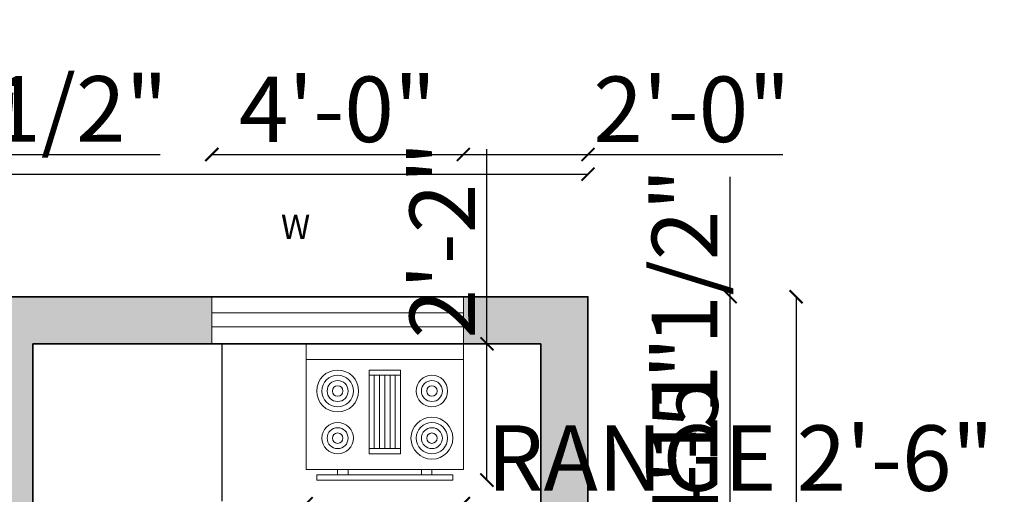
# Model space of a CAD drawing. Units: inches. Extents: x 1750 to 7466, y 1409 to 2004.
# Tile 5 of 5: x 1986 to 2174, y 1890 to 1981. Entities that reach past the tile are written whole.
import ezdxf

# ---------------------------------------------------------------- set-up
doc = ezdxf.new("R2010")
doc.units = ezdxf.units.IN
for name, color, linetype, lineweight in [('A-ANNO-DIMS', 2, 'Continuous', 18), ('A-ANNO-TEXT', 7, 'Continuous', 18), ('A-EQPM', 9, 'Continuous', 18), ('A-FLOR-CASE', 8, 'Continuous', 25), ('A-WALL', 7, 'Continuous', 35), ('WINDOW', 4, 'Continuous', 18)]:
    doc.layers.add(name, color=color, linetype=linetype, lineweight=lineweight)
doc.layers.add('A-WALL-PATT', color=18, linetype='Continuous', lineweight=13, true_color=0x000000)
doc.styles.get("Standard").update_dxf_attribs({"font": 'arial.ttf'})
doc.dimstyles.new('ISO-25', dxfattribs={"dimtxt": 12.5, "dimasz": 2.5, "dimexe": 1.25, "dimexo": 0.625, "dimtad": 1, "dimdec": 0, "dimlunit": 4, "dimtxsty": 'Standard', "dimblk": 'ARCHTICK', "dimcen": 2.5, "dimse1": 1, "dimse2": 1, "dimclrd": 2, "dimadec": 0, "dimazin": 0, "dimtfac": 1, "dimtdec": 0, "dimtmove": 0, "dimatfit": 3, "dimfxl": 1, "dimarcsym": 0})

# ---------------------------------------------------------------- blocks, each defined once
blk = doc.blocks.new('Range-Oven - 30 in top')
for p, q in [((0, -3), (30, -3)), ((12, -6), (18, -6)), ((13, -20), (13, -6)), ((14, -6), (14, -20)), ((15, -20), (15, -6)), ((16, -6), (16, -20)), ((17, -20), (17, -6)), ((18, -20), (12, -20)), ((6, -24), (6, -25)), ((8, -25), (8, -24)), ((22, -25), (22, -24)), ((24, -24), (24, -25))]:
    blk.add_line(p, q)
for points in [[(0, -24), (0, 0), (30, 0), (30, -24)], [(12, -21), (12, -5), (18, -5), (18, -21)], [(2, -26), (2, -25), (28, -25), (28, -26)]]:
    blk.add_lwpolyline(points, close=True)
for centre, radius in [((6, -9), 4), ((6, -9), 3), ((6, -9), 2), ((24, -9), 3), ((24, -9), 2), ((6, -9), 1), ((24, -9), 1), ((6, -18), 3), ((24, -18), 4), ((24, -18), 3), ((6, -18), 2), ((24, -18), 2), ((6, -18), 1), ((24, -18), 1)]:
    blk.add_circle(centre, radius)
blk = doc.blocks.new('_ArchTick')
at = {"color": 0, "linetype": 'ByBlock', "const_width": 0.15}
blk.add_lwpolyline([(-0.5, -0.5), (0.5, 0.5)], dxfattribs=at)
blk = doc.blocks.new('*D13')
at = {"layer": 'A-ANNO-DIMS', "color": 0, "lineweight": -2, "transparency": 16777216}
blk.add_line((1854.13, 1951.57), (2094.13, 1951.57), dxfattribs=at)
at = {"layer": 'Defpoints', "color": 0, "transparency": 16777216}
for p in [(2094.13, 1951.57), (1854.13, 1928.17), (2094.13, 1928.17)]:
    blk.add_point(p, dxfattribs=at)
at = {"layer": 'A-ANNO-DIMS', "color": 0, "lineweight": -2, "transparency": 16777216, "xscale": 2.5, "yscale": 2.5, "zscale": 2.5, "rotation": 180}
blk.add_blockref('_ArchTick', (1854.13, 1951.57), dxfattribs=at)
at = {"layer": 'A-ANNO-DIMS', "color": 0, "lineweight": -2, "transparency": 16777216, "xscale": 2.5, "yscale": 2.5, "zscale": 2.5}
blk.add_blockref('_ArchTick', (2094.13, 1951.57), dxfattribs=at)
at = {"layer": 'A-ANNO-DIMS', "color": 0, "transparency": 16777216, "insert": (1974.13, 1958.58), "char_height": 12.5, "attachment_point": 5}
blk.add_mtext("20'", dxfattribs=at)
blk = doc.blocks.new('*D14')
at = {"layer": 'A-ANNO-DIMS', "color": 0, "lineweight": -2, "transparency": 16777216}
blk.add_line((2133.87, 1928.17), (2133.87, 1448.17), dxfattribs=at)
at = {"layer": 'Defpoints', "color": 0, "transparency": 16777216}
for p in [(2094.13, 1928.17), (2094.13, 1448.17), (2133.87, 1448.17)]:
    blk.add_point(p, dxfattribs=at)
at = {"layer": 'A-ANNO-DIMS', "color": 0, "lineweight": -2, "transparency": 16777216, "xscale": 2.5, "yscale": 2.5, "zscale": 2.5}
for p, rotation in [((2133.87, 1928.17), 90), ((2133.87, 1448.17), 270)]:
    blk.add_blockref('_ArchTick', p, dxfattribs=dict(at, rotation=rotation))
at = {"layer": 'A-ANNO-DIMS', "color": 0, "transparency": 16777216, "insert": (2126.86, 1688.17), "char_height": 12.5, "attachment_point": 5, "rotation": 90}
blk.add_mtext("40'", dxfattribs=at)
blk = doc.blocks.new('*D19')
at = {"layer": 'A-ANNO-DIMS', "color": 2, "lineweight": -2, "transparency": 16777216}
for p, q in [((2040.34, 1888.67), (2070.34, 1888.67)), ((2070.34, 1888.67), (2173.62, 1888.67))]:
    blk.add_line(p, q, dxfattribs=at)
at = {"layer": 'Defpoints', "color": 0, "transparency": 16777216}
for p in [(2040.34, 1893.17), (2070.34, 1893.17), (2070.34, 1888.67)]:
    blk.add_point(p, dxfattribs=at)
at = {"layer": 'A-ANNO-DIMS', "color": 2, "lineweight": -2, "transparency": 16777216, "xscale": 2.5, "yscale": 2.5, "zscale": 2.5, "rotation": 180}
blk.add_blockref('_ArchTick', (2040.34, 1888.67), dxfattribs=at)
at = {"layer": 'A-ANNO-DIMS', "color": 2, "lineweight": -2, "transparency": 16777216, "xscale": 2.5, "yscale": 2.5, "zscale": 2.5}
blk.add_blockref('_ArchTick', (2070.34, 1888.67), dxfattribs=at)
at = {"layer": 'A-ANNO-DIMS', "color": 0, "transparency": 16777216, "insert": (2123.23, 1895.75), "char_height": 12.5, "attachment_point": 5}
blk.add_mtext('RANGE 2\'-6"', dxfattribs=at)
blk = doc.blocks.new('*D20')
at = {"layer": 'A-ANNO-DIMS', "color": 2, "lineweight": -2, "transparency": 16777216}
for p, q in [((2074.84, 1919.17), (2074.84, 1956.36)), ((2074.84, 1893.17), (2074.84, 1919.17))]:
    blk.add_line(p, q, dxfattribs=at)
at = {"layer": 'Defpoints', "color": 0, "transparency": 16777216}
for p in [(2070.34, 1919.17), (2074.84, 1919.17), (2070.34, 1893.17)]:
    blk.add_point(p, dxfattribs=at)
at = {"layer": 'A-ANNO-DIMS', "color": 2, "lineweight": -2, "transparency": 16777216, "xscale": 2.5, "yscale": 2.5, "zscale": 2.5}
for p, rotation in [((2074.84, 1919.17), 90), ((2074.84, 1893.17), 270)]:
    blk.add_blockref('_ArchTick', p, dxfattribs=dict(at, rotation=rotation))
at = {"layer": 'A-ANNO-DIMS', "color": 0, "transparency": 16777216, "insert": (2067.94, 1939.01), "char_height": 12.5, "attachment_point": 5, "rotation": 90}
blk.add_mtext('2\'-2"', dxfattribs=at)
blk = doc.blocks.new('*D39')
at = {"layer": 'A-ANNO-DIMS', "color": 2, "lineweight": -2, "transparency": 16777216}
for p, q in [((1775.98, 1919.17), (1775.98, 1889.13)), ((1775.98, 1889.13), (1775.98, 1851.94))]:
    blk.add_line(p, q, dxfattribs=at)
at = {"layer": 'Defpoints', "color": 0, "transparency": 16777216}
for p in [(2024.28, 1919.17), (1775.98, 1889.13), (2024.28, 1889.13)]:
    blk.add_point(p, dxfattribs=at)
at = {"layer": 'A-ANNO-DIMS', "color": 2, "lineweight": -2, "transparency": 16777216, "xscale": 2.5, "yscale": 2.5, "zscale": 2.5}
for p, rotation in [((1775.98, 1919.17), 90), ((1775.98, 1889.13), 270)]:
    blk.add_blockref('_ArchTick', p, dxfattribs=dict(at, rotation=rotation))
at = {"layer": 'A-ANNO-DIMS', "color": 0, "transparency": 16777216, "insert": (1768.98, 1869.28), "char_height": 12.5, "attachment_point": 5, "rotation": 90}
blk.add_mtext('2\'-6"', dxfattribs=at)
blk = doc.blocks.new('*D42')
at = {"layer": 'A-ANNO-DIMS', "color": 2, "lineweight": -2, "transparency": 16777216}
blk.add_line((2022.32, 1955.32), (2070.34, 1955.32), dxfattribs=at)
at = {"layer": 'Defpoints', "color": 0, "transparency": 16777216}
for p in [(2070.34, 1955.32), (2022.32, 1928.17), (2070.34, 1928.17)]:
    blk.add_point(p, dxfattribs=at)
at = {"layer": 'A-ANNO-DIMS', "color": 2, "lineweight": -2, "transparency": 16777216, "xscale": 2.5, "yscale": 2.5, "zscale": 2.5, "rotation": 180}
blk.add_blockref('_ArchTick', (2022.32, 1955.32), dxfattribs=at)
at = {"layer": 'A-ANNO-DIMS', "color": 2, "lineweight": -2, "transparency": 16777216, "xscale": 2.5, "yscale": 2.5, "zscale": 2.5}
blk.add_blockref('_ArchTick', (2070.34, 1955.32), dxfattribs=at)
at = {"layer": 'A-ANNO-DIMS', "color": 0, "transparency": 16777216, "insert": (2046.33, 1962.32), "char_height": 12.5, "attachment_point": 5}
blk.add_mtext('4\'-0"', dxfattribs=at)
blk = doc.blocks.new('*D43')
at = {"layer": 'A-ANNO-DIMS', "color": 2, "lineweight": -2, "transparency": 16777216}
for p, q in [((2070.34, 1955.32), (2094.13, 1955.32)), ((2094.13, 1955.32), (2131.32, 1955.32))]:
    blk.add_line(p, q, dxfattribs=at)
at = {"layer": 'Defpoints', "color": 0, "transparency": 16777216}
for p in [(2094.13, 1955.32), (2070.34, 1928.17), (2094.13, 1928.17)]:
    blk.add_point(p, dxfattribs=at)
at = {"layer": 'A-ANNO-DIMS', "color": 2, "lineweight": -2, "transparency": 16777216, "xscale": 2.5, "yscale": 2.5, "zscale": 2.5, "rotation": 180}
blk.add_blockref('_ArchTick', (2070.34, 1955.32), dxfattribs=at)
at = {"layer": 'A-ANNO-DIMS', "color": 2, "lineweight": -2, "transparency": 16777216, "xscale": 2.5, "yscale": 2.5, "zscale": 2.5}
blk.add_blockref('_ArchTick', (2094.13, 1955.32), dxfattribs=at)
at = {"layer": 'A-ANNO-DIMS', "color": 0, "transparency": 16777216, "insert": (2113.98, 1962.32), "char_height": 12.5, "attachment_point": 5}
blk.add_mtext('2\'-0"', dxfattribs=at)
blk = doc.blocks.new('*D44')
at = {"layer": 'A-ANNO-DIMS', "color": 2, "lineweight": -2, "transparency": 16777216}
for p, q in [((2121.28, 1875.24), (2121.28, 1951.04)), ((2121.28, 1827.64), (2121.28, 1875.24))]:
    blk.add_line(p, q, dxfattribs=at)
at = {"layer": 'Defpoints', "color": 0, "transparency": 16777216}
for p in [(2094.13, 1875.24), (2121.28, 1875.24), (2094.13, 1827.64)]:
    blk.add_point(p, dxfattribs=at)
at = {"layer": 'A-ANNO-DIMS', "color": 2, "lineweight": -2, "transparency": 16777216, "xscale": 2.5, "yscale": 2.5, "zscale": 2.5}
for p, rotation in [((2121.28, 1875.24), 90), ((2121.28, 1827.64), 270)]:
    blk.add_blockref('_ArchTick', p, dxfattribs=dict(at, rotation=rotation))
at = {"layer": 'A-ANNO-DIMS', "color": 0, "transparency": 16777216, "insert": (2114.19, 1914.39), "char_height": 12.5, "attachment_point": 5, "rotation": 90}
blk.add_mtext('3\'-11 1/2"', dxfattribs=at)
blk = doc.blocks.new('*D45')
at = {"layer": 'A-ANNO-DIMS', "color": 2, "lineweight": -2, "transparency": 16777216}
blk.add_line((2121.28, 1875.24), (2121.28, 1928.17), dxfattribs=at)
at = {"layer": 'Defpoints', "color": 0, "transparency": 16777216}
for p in [(2094.13, 1928.17), (2121.28, 1928.17), (2094.13, 1875.24)]:
    blk.add_point(p, dxfattribs=at)
at = {"layer": 'A-ANNO-DIMS', "color": 2, "lineweight": -2, "transparency": 16777216, "xscale": 2.5, "yscale": 2.5, "zscale": 2.5}
for p, rotation in [((2121.28, 1928.17), 90), ((2121.28, 1875.24), 270)]:
    blk.add_blockref('_ArchTick', p, dxfattribs=dict(at, rotation=rotation))
at = {"layer": 'A-ANNO-DIMS', "color": 0, "transparency": 16777216, "insert": (2114.3, 1901.7), "char_height": 12.5, "attachment_point": 5, "rotation": 90}
blk.add_mtext('4\'-5"', dxfattribs=at)
blk = doc.blocks.new('*D47')
at = {"layer": 'A-ANNO-DIMS', "color": 2, "lineweight": -2, "transparency": 16777216}
for p, q in [((1775.98, 1928.17), (1775.98, 1919.17)), ((1775.98, 1919.17), (1775.98, 1882.19))]:
    blk.add_line(p, q, dxfattribs=at)
at = {"layer": 'Defpoints', "color": 0, "transparency": 16777216}
for p in [(2022.32, 1928.17), (1775.98, 1919.17), (2022.32, 1919.17)]:
    blk.add_point(p, dxfattribs=at)
at = {"layer": 'A-ANNO-DIMS', "color": 2, "lineweight": -2, "transparency": 16777216, "xscale": 2.5, "yscale": 2.5, "zscale": 2.5}
for p, rotation in [((1775.98, 1928.17), 90), ((1775.98, 1919.17), 270)]:
    blk.add_blockref('_ArchTick', p, dxfattribs=dict(at, rotation=rotation))
at = {"layer": 'A-ANNO-DIMS', "color": 0, "transparency": 16777216, "insert": (1768.98, 1899.43), "char_height": 12.5, "attachment_point": 5, "rotation": 90}
blk.add_mtext('0\'-9"', dxfattribs=at)
blk = doc.blocks.new('*D50')
at = {"layer": 'A-ANNO-DIMS', "color": 2, "lineweight": -2, "transparency": 16777216}
for p, q in [((1896.49, 1955.32), (1945.82, 1955.32)), ((1945.82, 1955.32), (2012.43, 1955.32))]:
    blk.add_line(p, q, dxfattribs=at)
at = {"layer": 'Defpoints', "color": 0, "transparency": 16777216}
for p in [(1945.82, 1955.32), (1896.49, 1928.17), (1945.82, 1928.17)]:
    blk.add_point(p, dxfattribs=at)
at = {"layer": 'A-ANNO-DIMS', "color": 2, "lineweight": -2, "transparency": 16777216, "xscale": 2.5, "yscale": 2.5, "zscale": 2.5, "rotation": 180}
blk.add_blockref('_ArchTick', (1896.49, 1955.32), dxfattribs=at)
at = {"layer": 'A-ANNO-DIMS', "color": 2, "lineweight": -2, "transparency": 16777216, "xscale": 2.5, "yscale": 2.5, "zscale": 2.5}
blk.add_blockref('_ArchTick', (1945.82, 1955.32), dxfattribs=at)
at = {"layer": 'A-ANNO-DIMS', "color": 0, "transparency": 16777216, "insert": (1980.37, 1962.4), "char_height": 12.5, "attachment_point": 5}
blk.add_mtext('4\'-1 1/2"', dxfattribs=at)
blk = doc.blocks.new('*D55')
at = {"layer": 'A-ANNO-DIMS', "color": 2, "lineweight": -2, "transparency": 16777216}
blk.add_line((1775.98, 1928.17), (1775.98, 1799.17), dxfattribs=at)
at = {"layer": 'Defpoints', "color": 0, "transparency": 16777216}
for p in [(2022.32, 1928.17), (1775.98, 1799.17), (1995.93, 1799.17)]:
    blk.add_point(p, dxfattribs=at)
at = {"layer": 'A-ANNO-DIMS', "color": 2, "lineweight": -2, "transparency": 16777216, "xscale": 2.5, "yscale": 2.5, "zscale": 2.5}
for p, rotation in [((1775.98, 1928.17), 90), ((1775.98, 1799.17), 270)]:
    blk.add_blockref('_ArchTick', p, dxfattribs=dict(at, rotation=rotation))
at = {"layer": 'A-ANNO-DIMS', "color": 0, "transparency": 16777216, "insert": (1768.98, 1863.67), "char_height": 12.5, "attachment_point": 5, "rotation": 90}
blk.add_mtext('10\'-9"', dxfattribs=at)

msp = doc.modelspace()

# ---------------------------------------------------------------- hatches: boundary and pattern name
at = {"layer": 'A-WALL-PATT'}
h = msp.add_hatch(color=256, dxfattribs=at)
h.dxf.hatch_style = 1
h.paths.add_polyline_path([(1896.49, 1928.17), (1854.13, 1928.17), (1854.13, 1893.52), (1863.13, 1893.52), (1863.13, 1919.17), (1896.49, 1919.17)])
h.paths.add_polyline_path([(2022.32, 1928.17), (1945.82, 1928.17), (1945.82, 1919.17), (1983.13, 1919.17), (1983.13, 1804.17), (1974.13, 1804.17), (1974.13, 1799.17), (1995.93, 1799.17), (1995.93, 1804.17), (1988.13, 1804.17), (1988.13, 1919.17), (2022.32, 1919.17)])
h.paths.add_polyline_path([(2094.13, 1928.17), (2070.34, 1928.17), (2070.34, 1919.17), (2085.13, 1919.17), (2085.13, 1875.24), (2094.13, 1875.24)])
h.paths.add_polyline_path([(2094.13, 1827.64), (2085.13, 1827.64), (2085.13, 1804.17), (2035.93, 1804.17), (2035.93, 1799.17), (2085.13, 1799.17), (2085.13, 1763.18), (2094.13, 1763.18)])
h.paths.add_polyline_path([(1863.13, 1846.52), (1854.13, 1846.52), (1854.13, 1751.88), (1863.13, 1751.88)])
h.paths.add_polyline_path([(1934.13, 1804.17), (1863.13, 1804.17), (1863.13, 1799.17), (1911.13, 1799.17), (1911.13, 1794.68), (1912.55, 1794.68), (1916.13, 1794.68), (1916.13, 1799.17), (1934.13, 1799.17)])
h.paths.add_polyline_path([(1863.13, 1726.23), (1854.13, 1726.23), (1854.13, 1709.82), (1863.13, 1709.82), (1863.13, 1714.17), (1911.13, 1714.17), (1911.13, 1671.17), (1887.9, 1671.17, -0.01479), (1887.95, 1669.75), (1887.95, 1666.17), (1916.13, 1666.17), (1940.64, 1666.17), (1940.64, 1671.17), (1916.13, 1671.17), (1916.13, 1770.77), (1912.55, 1770.77, -0.01479), (1911.13, 1770.81), (1911.13, 1719.17), (1863.13, 1719.17)])
h.paths.add_polyline_path([(1863.13, 1684.17), (1854.13, 1684.17), (1854.13, 1625.24), (1863.13, 1625.24)])
h.paths.add_polyline_path([(1863.13, 1577.33), (1854.13, 1577.33), (1854.13, 1526.31), (1863.13, 1526.31), (1863.13, 1544.17), (1983.13, 1544.17), (1988.13, 1544.17), (1990.13, 1544.17), (1990.13, 1549.17), (1990.13, 1620.17), (1996.77, 1620.17), (1996.77, 1625.17), (1990.13, 1625.17), (1990.13, 1666.17), (1990.13, 1671.17), (1980.64, 1671.17), (1980.64, 1666.17), (1985.13, 1666.17), (1985.13, 1625.17), (1985.13, 1549.17), (1863.13, 1549.17)])
h.paths.add_polyline_path([(1988.13, 1457.17), (1863.13, 1457.17), (1863.13, 1497.36), (1854.13, 1497.36), (1854.13, 1448.17), (1988.13, 1448.17)])
h.paths.add_polyline_path([(2031.23, 1454.78), (1988.13, 1454.78), (1988.13, 1450.91), (2031.23, 1450.91)])
h.paths.add_polyline_path([(2074.33, 1454.78), (2037.79, 1454.78), (2037.79, 1450.91), (2074.33, 1450.91)], flags=17)
h.paths.add_polyline_path([(2094.13, 1714.84), (2085.13, 1714.84), (2085.13, 1625.17), (2036.77, 1625.17), (2036.77, 1620.17), (2085.13, 1620.17), (2085.13, 1457.17), (2074.33, 1457.17), (2074.33, 1448.17), (2094.13, 1448.17)])
h.paths.add_polyline_path([(1846.92, 1867), (1855.4, 1867), (1855.4, 1874), (1846.92, 1874)], flags=9)
h.paths.add_polyline_path([(1885.75, 1686.15), (1909.97, 1686.15), (1909.97, 1693.31), (1885.75, 1693.31)], flags=25)
h.paths.add_polyline_path([(1885.73, 1693.64), (1900.82, 1693.64), (1900.82, 1700.88), (1885.73, 1700.88)], flags=25)
h.paths.add_polyline_path([(1866.42, 1762.99), (1892.45, 1762.99), (1892.45, 1770.14), (1866.42, 1770.14)], flags=25)
h.paths.add_polyline_path([(1866.4, 1770.47), (1898.87, 1770.47), (1898.87, 1777.71), (1866.4, 1777.71)], flags=9)
h.paths.add_polyline_path([(1925.02, 1731.07), (1964.24, 1731.07), (1964.24, 1738.22), (1925.02, 1738.22)], flags=9)
h.paths.add_polyline_path([(1925.01, 1738.55), (1982.11, 1738.55), (1982.11, 1745.79), (1925.01, 1745.79)], flags=9)
h.paths.add_polyline_path([(1995.48, 1862.99), (2034.71, 1862.99), (2034.71, 1870.14), (1995.48, 1870.14)], flags=9)
h.paths.add_polyline_path([(1995.47, 1870.47), (2026.49, 1870.47), (2026.49, 1877.71), (1995.47, 1877.71)], flags=9)
h.paths.add_polyline_path([(1869.07, 1829.02), (1905.98, 1829.02), (1905.98, 1836.17), (1869.07, 1836.17)], flags=9)
h.paths.add_polyline_path([(1869.05, 1836.5), (1905.15, 1836.5), (1905.15, 1843.74), (1869.05, 1843.74)], flags=9)

# ---------------------------------------------------------------- linework, layer by layer
at = {"layer": 'A-FLOR-CASE'}
msp.add_line((2024.28, 1889.13), (2024.28, 1919.17), dxfattribs=at)
at = {"layer": 'A-WALL'}
for p, q in [((1988.13, 1804.17), (1988.13, 1919.17)), ((1988.13, 1919.17), (2085.13, 1919.17)), ((2085.13, 1919.17), (2085.13, 1804.17))]:
    msp.add_line(p, q, dxfattribs=at)
msp.add_lwpolyline([(1988.13, 1448.17), (1854.13, 1448.17), (1854.13, 1928.17), (2094.13, 1928.17), (2094.13, 1448.17), (2074.33, 1448.17)], dxfattribs=at)
at = {"layer": 'WINDOW'}
for p, q in [((2022.32, 1928.17), (2022.32, 1919.17)), ((2070.34, 1928.17), (2022.32, 1928.17)), ((2070.34, 1919.17), (2070.34, 1928.17)), ((2070.34, 1925.11), (2022.32, 1925.11)), ((2070.34, 1922.43), (2022.32, 1922.43)), ((2022.32, 1919.17), (2070.34, 1919.17))]:
    msp.add_line(p, q, dxfattribs=at)

# ---------------------------------------------------------------- block references
at = {"layer": 'A-EQPM'}
msp.add_blockref('Range-Oven - 30 in top', (2040.34, 1919.17), dxfattribs=at)

# ---------------------------------------------------------------- texts
at = {"layer": 'A-ANNO-TEXT'}
msp.add_text('W', height=4.67, dxfattribs=at).set_placement((2035.51, 1939.18))

# ---------------------------------------------------------------- dimensions: what is measured, and where the dimension line sits
at = {"layer": 'A-ANNO-DIMS'}
for base, p1, p2, override, picture, middle in [((1945.82, 1955.32), (1896.49, 1928.17), (1945.82, 1928.17), {"dimdec": 1, "dimlfac": 1, "dimrnd": 0, "dimzin": 1, "dimdsep": 46, "dimlunit": 4, "dimfrac": 2}, '*D50', (1980.37, 1962.4)), ((2070.34, 1955.32), (2022.32, 1928.17), (2070.34, 1928.17), {"dimdec": 1, "dimlfac": 1, "dimrnd": 0, "dimzin": 1, "dimdsep": 46, "dimlunit": 4, "dimfrac": 2}, '*D42', (2046.33, 1962.32)), ((2094.13, 1955.32), (2070.34, 1928.17), (2094.13, 1928.17), {"dimdec": 1, "dimlfac": 1, "dimrnd": 0, "dimzin": 1, "dimdsep": 46, "dimlunit": 4, "dimfrac": 2}, '*D43', (2113.98, 1962.32)), ((2094.13, 1951.57), (1854.13, 1928.17), (2094.13, 1928.17), {"dimclrd": 0, "dimclre": 0, "dimclrt": 0}, '*D13', (1974.13, 1958.58))]:
    dim = msp.add_linear_dim(base=base, p1=p1, p2=p2, dimstyle='ISO-25', override=override, dxfattribs=at)
    dim.commit()
    dim.dimension.update_dxf_attribs({"geometry": picture, "text_midpoint": middle})
for base, p1, p2, override, picture, middle in [((2074.84, 1919.17), (2070.34, 1893.17), (2070.34, 1919.17), {"dimdec": 1, "dimlfac": 1, "dimrnd": 0, "dimzin": 1, "dimdsep": 46, "dimlunit": 4, "dimfrac": 2}, '*D20', (2067.94, 1939.01)), ((2121.28, 1875.24), (2094.13, 1827.64), (2094.13, 1875.24), {"dimdec": 1, "dimlfac": 1, "dimrnd": 0, "dimzin": 1, "dimdsep": 46, "dimlunit": 4, "dimfrac": 2}, '*D44', (2114.19, 1914.39)), ((1775.98, 1919.17), (2022.32, 1928.17), (2022.32, 1919.17), {"dimdec": 1, "dimlfac": 1, "dimrnd": 0, "dimzin": 1, "dimdsep": 46, "dimlunit": 4, "dimfrac": 2}, '*D47', (1768.98, 1899.43)), ((1775.98, 1799.17), (2022.32, 1928.17), (1995.93, 1799.17), {"dimdec": 1, "dimlfac": 1, "dimrnd": 0, "dimzin": 1, "dimdsep": 46, "dimlunit": 4, "dimfrac": 2}, '*D55', (1768.98, 1863.67)), ((2133.87, 1448.17), (2094.13, 1928.17), (2094.13, 1448.17), {"dimclrd": 0, "dimclre": 0, "dimclrt": 0}, '*D14', (2126.86, 1688.17)), ((2121.28, 1928.17), (2094.13, 1875.24), (2094.13, 1928.17), {"dimdec": 1, "dimlfac": 1, "dimrnd": 0, "dimzin": 1, "dimdsep": 46, "dimlunit": 4, "dimfrac": 2}, '*D45', (2114.3, 1901.7)), ((1775.98, 1889.13), (2024.28, 1919.17), (2024.28, 1889.13), {"dimdec": 1, "dimlfac": 1, "dimrnd": 0, "dimzin": 1, "dimdsep": 46, "dimlunit": 4, "dimfrac": 2}, '*D39', (1768.98, 1869.28))]:
    dim = msp.add_linear_dim(base=base, p1=p1, p2=p2, angle=90, dimstyle='ISO-25', override=override, dxfattribs=at)
    dim.commit()
    dim.dimension.update_dxf_attribs({"geometry": picture, "text_midpoint": middle})
dim = msp.add_linear_dim(base=(2070.34, 1888.67), p1=(2040.34, 1893.17), p2=(2070.34, 1893.17), text='RANGE <>', dimstyle='ISO-25', override={"dimdec": 1, "dimlfac": 1, "dimrnd": 0, "dimzin": 1, "dimdsep": 46, "dimlunit": 4, "dimfrac": 2}, dxfattribs=at)
dim.commit()
dim.dimension.update_dxf_attribs({"geometry": '*D19', "text_midpoint": (2123.23, 1895.75)})

doc.saveas('drawing.dxf')
